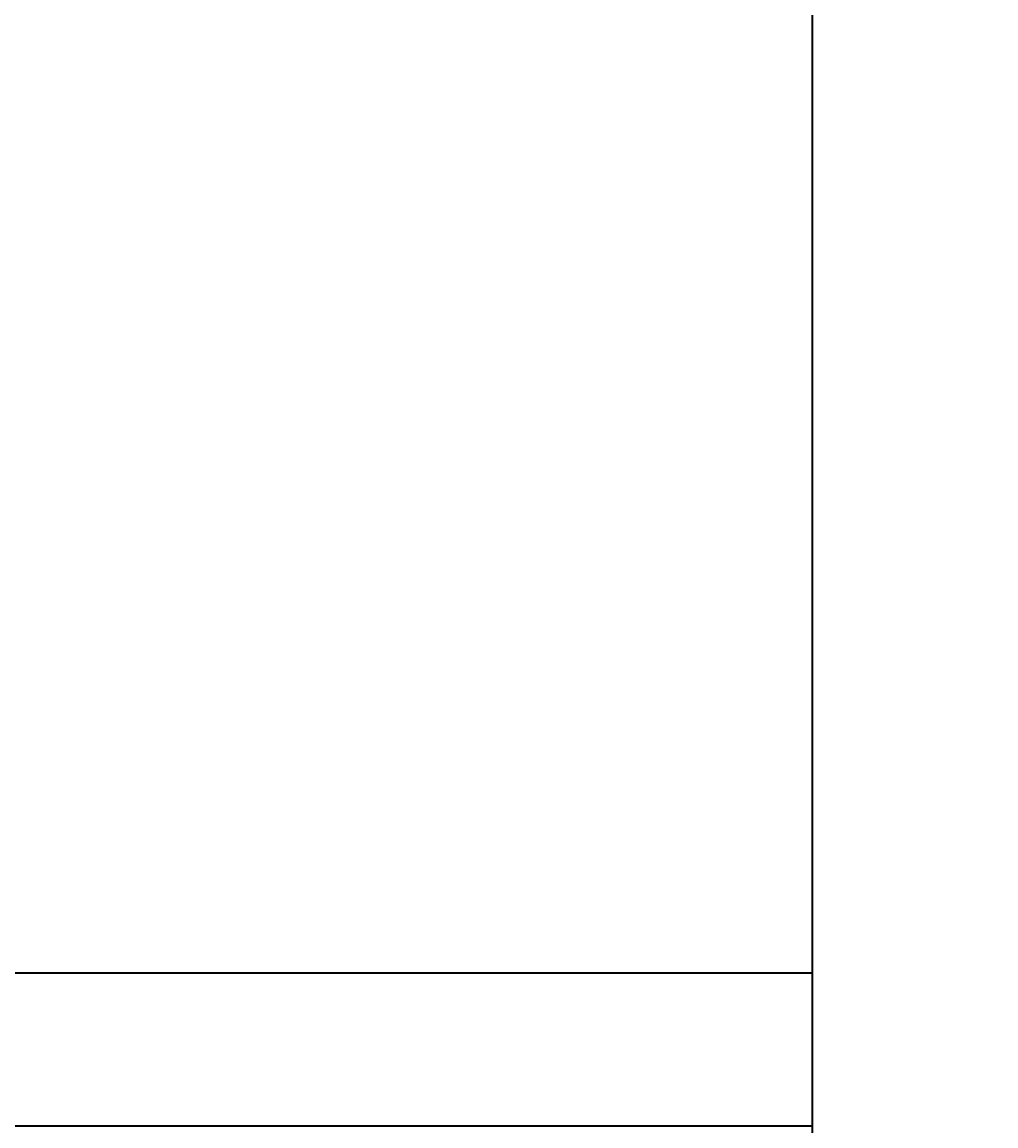
# Model space of a CAD drawing. Units: millimetres. Extents: x 27017497 to 27018854, y 7058029 to 7059154.
# Tile 54 of 91: x 27018009 to 27018038, y 7058294 to 7058327. Entities that reach past the tile are written whole.
import ezdxf

# ---------------------------------------------------------------- set-up
doc = ezdxf.new("R2010")
doc.units = ezdxf.units.MM
doc.layers.add('A-ANNO-DIMS', color=2, linetype='Continuous', lineweight=18)
doc.layers.add('A-WALL', color=7, linetype='Continuous', lineweight=35)
doc.styles.get("Standard").update_dxf_attribs({"font": 'arial.ttf'})
doc.dimstyles.get("Standard").update_dxf_attribs({"dimtxt": 0.18, "dimasz": 0.18, "dimexe": 0.18, "dimexo": 0.0625, "dimgap": 0.09, "dimtad": 0, "dimtih": 1, "dimtoh": 1, "dimdec": 4, "dimzin": 0, "dimdsep": 46, "dimtxsty": 'Standard', "dimcen": 0.09, "dimadec": 0, "dimazin": 0, "dimtfac": 1, "dimtdec": 4, "dimtofl": 0, "dimtmove": 0, "dimatfit": 3, "dimfxl": 1, "dimtolj": 1, "dimtzin": 0, "dimarcsym": 0})

# ---------------------------------------------------------------- blocks, each defined once
blk = doc.blocks.new('*D48')
at = {"layer": 'A-ANNO-DIMS', "color": 0, "lineweight": -2, "transparency": 16777216}
for p, q in [((27018463.498, 7058622.912), (27017497.536, 7058622.912)), ((27017497.716, 7058622.732), (27017497.716, 7058357.753)), ((27017497.716, 7058092.41), (27017497.716, 7058357.389)), ((27018555.129, 7058092.23), (27017497.536, 7058092.23))]:
    blk.add_line(p, q, dxfattribs=at)
at = {"layer": 'A-ANNO-DIMS', "color": 0, "transparency": 16777216}
for points in [[(27017497.686, 7058622.732), (27017497.746, 7058622.732), (27017497.716, 7058622.912)], [(27017497.686, 7058092.41), (27017497.746, 7058092.41), (27017497.716, 7058092.23)]]:
    blk.add_solid(points, dxfattribs=at)
at = {"layer": 'Defpoints', "color": 0, "transparency": 16777216}
for p in [(27018463.561, 7058622.912), (27017497.716, 7058092.23), (27018555.192, 7058092.23)]:
    blk.add_point(p, dxfattribs=at)
at = {"layer": 'A-ANNO-DIMS', "color": 0, "transparency": 16777216, "insert": (27017497.716, 7058357.571), "char_height": 0.18, "attachment_point": 5}
blk.add_mtext('\\A1;530.7', dxfattribs=at)

msp = doc.modelspace()

# ---------------------------------------------------------------- linework, layer by layer
at = {"layer": 'A-WALL'}
for p, q in [((27018032.166, 7058386.803), (27018032.166, 7058141.912)), ((27017888.166, 7058298.912), (27018032.166, 7058298.912)), ((27017888.166, 7058294.412), (27018032.166, 7058294.412))]:
    msp.add_line(p, q, dxfattribs=at)
msp.add_lwpolyline([(27018032.178, 7058237.363), (27018032.178, 7058375.363)], dxfattribs=at)

# ---------------------------------------------------------------- dimensions: what is measured, and where the dimension line sits
at = {"layer": 'A-ANNO-DIMS'}
dim = msp.add_linear_dim(base=(27017497.716, 7058092.23), p1=(27018463.561, 7058622.912), p2=(27018555.192, 7058092.23), angle=90, dimstyle='Standard', override={"dimdec": 1, "dimlfac": 1, "dimrnd": 0, "dimzin": 0, "dimdsep": 46, "dimlunit": 2}, dxfattribs=at)
dim.commit()
dim.dimension.update_dxf_attribs({"geometry": '*D48', "text_midpoint": (27017497.716, 7058357.571)})

doc.saveas('drawing.dxf')
